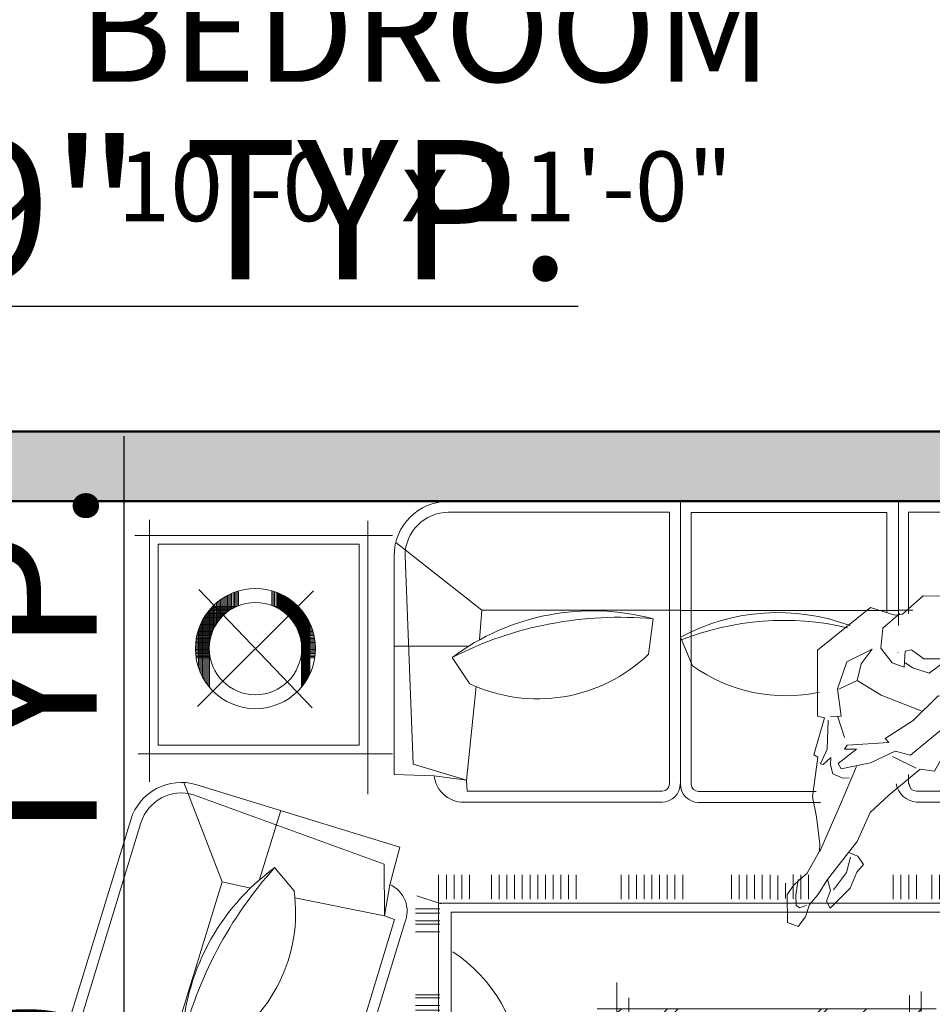
# Model space of a CAD drawing. Units: inches. Extents: x 375 to 1122, y 27 to 1069.
# Tile 75 of 155: x 509 to 588, y 792 to 877. Entities that reach past the tile are written whole.
import ezdxf

# ---------------------------------------------------------------- set-up
doc = ezdxf.new("R2010")
doc.units = ezdxf.units.IN
for name, color, linetype, lineweight in [('A-ANNO-DIMS', 2, 'Continuous', 18), ('A-AREA-IDEN', 7, 'Continuous', 18), ('A-WALL-PATT', 252, 'Continuous', 13), ('Furniture', 30, 'Continuous', 18), ('Walls', 250, 'Continuous', 50)]:
    doc.layers.add(name, color=color, linetype=linetype, lineweight=lineweight)
doc.styles.get("Standard").update_dxf_attribs({"font": 'arial.ttf'})
doc.dimstyles.new('ISO-25', dxfattribs={"dimtxt": 12, "dimasz": 2.5, "dimexe": 1.5, "dimexo": 1.5, "dimtad": 1, "dimdec": 1, "dimlunit": 3, "dimtxsty": 'Standard', "dimblk": 'ARCHTICK', "dimcen": 2.5, "dimadec": 0, "dimazin": 0, "dimtfac": 1, "dimtdec": 1, "dimtmove": 0, "dimatfit": 3, "dimfxl": 1.5, "dimfxlon": 1, "dimarcsym": 0})

# ---------------------------------------------------------------- blocks, each defined once
blk = doc.blocks.new('A$C4DC51D13')
for p, q in [((3265.3, 2996.2), (1188.4, 2996.2)), ((1895.2, 2134), (1895.2, 2996.2)), ((2559.6, 2996.2), (2559.6, 2617.8)), ((1188.4, 2962.7), (1862.1, 2962.7)), ((1862.1, 2134), (1862.1, 2962.7)), ((1928.3, 2961.6), (2524.2, 2961.6)), ((1928.3, 2134), (1928.3, 2961.6)), ((2524.2, 2961.6), (2524.2, 2658.6)), ((2590.4, 2962.7), (2590.4, 2654.5)), ((3265.3, 2962.7), (2590.4, 2962.7)), ((277.4, 2939.6), (277.4, 2141.8)), ((943, 2103.5), (943, 2936.7)), ((1018.2, 2892.3), (232.2, 2892.3)), ((3778.5, 2897), (3631.2, 2747.3)), ((4008.9, 2375.5), (3778.5, 2897)), ((4156.2, 2525.2), (3778.5, 2897)), ((304, 2865.7), (304, 2253.3)), ((916.4, 2865.7), (304, 2865.7)), ((916.4, 2253.3), (916.4, 2865.7)), ((1290.4, 2664.8), (1028, 2870.9)), ((3163.3, 2664.8), (3425.7, 2870.9)), ((1022.9, 2163.8), (1022.9, 2830.3)), ((1056, 2830.3), (1081, 2194.8)), ((3397.7, 2830.3), (3364.5, 2194.8)), ((3430.8, 2163.8), (3430.8, 2830.3)), ((4008.9, 2375.5), (3631.2, 2747.3)), ((423.7, 2370.8), (776.6, 2723.7)), ((427.4, 2727.4), (772.8, 2367.1)), ((502.2, 2648.3), (502.2, 2701.8)), ((506.4, 2652.2), (506.4, 2704.4)), ((510.6, 2655.8), (510.6, 2706.9)), ((514.9, 2659.2), (514.9, 2709.2)), ((519.1, 2662.3), (519.1, 2711.3)), ((523.3, 2665.1), (523.3, 2713.4)), ((527.5, 2667.8), (527.5, 2715.2)), ((531.8, 2670.2), (531.8, 2717)), ((536, 2672.5), (536, 2718.7)), ((540.2, 2674.6), (540.2, 2720.2)), ((544.4, 2676.5), (544.4, 2721.6)), ((548.7, 2678.2), (548.7, 2722.9)), ((650.1, 2678.8), (650.1, 2723.3)), ((654.3, 2677.1), (654.3, 2722)), ((658.6, 2675.2), (658.6, 2720.7)), ((662.8, 2673.2), (662.8, 2719.2)), ((667, 2671), (667, 2717.6)), ((668.5, 2670.2), (668.5, 2717)), ((671.2, 2668.6), (671.2, 2715.9)), ((672.7, 2667.8), (672.7, 2715.2)), ((675.5, 2666.1), (675.5, 2714)), ((676.9, 2665.1), (676.9, 2713.4)), ((679.7, 2663.3), (679.7, 2712)), ((681.1, 2662.3), (681.1, 2711.3)), ((683.9, 2660.3), (683.9, 2709.9)), ((685.4, 2659.2), (685.4, 2709.2)), ((688.1, 2657), (688.1, 2707.7)), ((689.6, 2655.8), (689.6, 2706.9)), ((692.4, 2653.5), (692.4, 2705.3)), ((693.8, 2652.2), (693.8, 2704.4)), ((696.6, 2649.6), (696.6, 2702.7)), ((698, 2648.3), (698, 2701.8)), ((700.8, 2645.5), (700.8, 2700)), ((465.8, 2671.5), (534.1, 2671.5)), ((468.4, 2596.6), (468.4, 2674.3)), ((469.8, 2675.7), (542.8, 2675.7)), ((472.6, 2606.7), (472.6, 2678.5)), ((476.8, 2615), (476.8, 2682.5)), ((481, 2622.2), (481, 2686.2)), ((485.3, 2628.5), (485.3, 2689.7)), ((489.5, 2634.2), (489.5, 2693)), ((493.7, 2639.3), (493.7, 2696.1)), ((497.9, 2644), (497.9, 2699.1)), ((657.4, 2675.7), (730.4, 2675.7)), ((734.5, 2671.5), (666.1, 2671.5)), ((666.1, 2671.5), (734.5, 2671.5)), ((702.3, 2644), (702.3, 2699.1)), ((705, 2641), (705, 2697.2)), ((706.5, 2639.3), (706.5, 2696.1)), ((709.3, 2636), (709.3, 2694.1)), ((710.7, 2634.2), (710.7, 2693)), ((713.5, 2630.5), (713.5, 2690.9)), ((714.9, 2628.5), (714.9, 2689.7)), ((717.7, 2624.4), (717.7, 2687.4)), ((719.2, 2622.2), (719.2, 2686.2)), ((722, 2617.6), (722, 2683.8)), ((723.4, 2615), (723.4, 2682.5)), ((726.2, 2609.7), (726.2, 2679.9)), ((727.6, 2606.7), (727.6, 2678.5)), ((730.4, 2600.3), (730.4, 2675.7)), ((731.9, 2596.6), (731.9, 2674.3)), ((734.6, 2588.4), (734.6, 2671.3)), ((3631.7, 2676.6), (3938.2, 2375)), ((443, 2453.4), (443, 2641.1)), ((443.5, 2641.9), (496, 2641.9)), ((446.1, 2646.1), (500, 2646.1)), ((447.2, 2446.7), (447.2, 2647.8)), ((448.9, 2650.4), (504.4, 2650.4)), ((451.5, 2440.6), (451.5, 2654)), ((451.9, 2654.6), (509.2, 2654.6)), ((455.1, 2658.8), (514.4, 2658.8)), ((455.7, 2434.9), (455.7, 2659.6)), ((458.4, 2663.1), (520.2, 2663.1)), ((459.9, 2558.8), (459.9, 2664.9)), ((462, 2667.3), (526.7, 2667.3)), ((464.1, 2583.3), (464.1, 2669.7)), ((489.5, 2667.3), (489.5, 2633.5)), ((738.2, 2667.3), (673.5, 2667.3)), ((673.5, 2667.3), (738.2, 2667.3)), ((741.8, 2663.1), (680, 2663.1)), ((680, 2663.1), (741.8, 2663.1)), ((745.2, 2658.8), (685.8, 2658.8)), ((685.8, 2658.8), (745.2, 2658.8)), ((748.3, 2654.6), (691, 2654.6)), ((691, 2654.6), (748.3, 2654.6)), ((751.3, 2650.4), (695.8, 2650.4)), ((695.8, 2650.4), (751.3, 2650.4)), ((754.1, 2646.1), (700.2, 2646.1)), ((700.2, 2646.1), (754.1, 2646.1)), ((756.7, 2641.9), (704.2, 2641.9)), ((704.2, 2641.9), (756.7, 2641.9)), ((736.1, 2583.3), (736.1, 2669.7)), ((738.9, 2570.4), (738.9, 2666.6)), ((740.3, 2558.8), (740.3, 2664.9)), ((743.1, 2433.1), (743.1, 2661.5)), ((744.5, 2434.9), (744.5, 2659.6)), ((747.3, 2438.6), (747.3, 2656)), ((748.8, 2440.6), (748.8, 2654)), ((751.5, 2444.5), (751.5, 2650)), ((753, 2446.7), (753, 2647.8)), ((755.8, 2451.1), (755.8, 2643.5)), ((757.2, 2453.4), (757.2, 2641.1)), ((1283.3, 2574.2), (1290.4, 2664.8)), ((1290.4, 2664.8), (1894.7, 2664.8)), ((1895.2, 2663.7), (2557.3, 2663.7)), ((2603.6, 2664.8), (2559, 2664.8)), ((3163.3, 2664.8), (2764.7, 2664.8)), ((3170.4, 2574.2), (3163.3, 2664.8)), ((429.1, 2612.3), (475.4, 2612.3)), ((430.3, 2479), (430.3, 2615.5)), ((430.7, 2616.6), (477.7, 2616.6)), ((432.5, 2620.8), (480.2, 2620.8)), ((434.5, 2469.3), (434.5, 2625.2)), ((434.5, 2625), (482.9, 2625)), ((436.5, 2629.2), (485.8, 2629.2)), ((438.7, 2633.5), (488.9, 2633.5)), ((438.8, 2460.9), (438.8, 2633.6)), ((441, 2637.7), (492.3, 2637.7)), ((759.2, 2637.7), (707.9, 2637.7)), ((707.9, 2637.7), (759.2, 2637.7)), ((761.5, 2633.5), (711.3, 2633.5)), ((711.3, 2633.5), (761.5, 2633.5)), ((763.7, 2629.2), (714.4, 2629.2)), ((714.4, 2629.2), (763.7, 2629.2)), ((765.8, 2625), (717.3, 2625)), ((767.7, 2620.8), (720, 2620.8)), ((769.5, 2616.6), (722.5, 2616.6)), ((771.1, 2612.3), (724.8, 2612.3)), ((760, 2458.3), (760, 2636.3)), ((761.4, 2460.9), (761.4, 2633.6)), ((764.2, 2466.3), (764.2, 2628.2)), ((765.7, 2469.3), (765.7, 2625.2)), ((1798, 2530.2), (1812.1, 2637.9)), ((420.6, 2582.7), (464, 2582.7)), ((421.5, 2587), (465.2, 2587)), ((422.5, 2591.2), (466.5, 2591.2)), ((423.6, 2595.4), (467.9, 2595.4)), ((424.8, 2599.7), (469.6, 2599.7)), ((426.1, 2603.9), (471.3, 2603.9)), ((426.1, 2490.7), (426.1, 2603.9)), ((427.5, 2608.1), (473.3, 2608.1)), ((772.7, 2608.1), (726.9, 2608.1)), ((774.1, 2603.9), (728.9, 2603.9)), ((775.4, 2599.7), (730.7, 2599.7)), ((776.6, 2595.4), (732.3, 2595.4)), ((777.7, 2591.2), (733.7, 2591.2)), ((778.7, 2587), (735.1, 2587)), ((779.6, 2582.7), (736.2, 2582.7)), ((1895.5, 2582.2), (1932.3, 2494.6)), ((417.2, 2553.2), (459.6, 2553.2)), ((417.4, 2557.4), (459.8, 2557.4)), ((417.7, 2561.6), (460.2, 2561.6)), ((418.1, 2565.8), (460.7, 2565.8)), ((418.5, 2570.1), (461.3, 2570.1)), ((419.1, 2574.3), (462.1, 2574.3)), ((419.8, 2578.5), (462.9, 2578.5)), ((780.4, 2578.5), (737.3, 2578.5)), ((781.1, 2574.3), (738.2, 2574.3)), ((781.7, 2570.1), (738.9, 2570.1)), ((782.2, 2565.8), (739.6, 2565.8)), ((782.5, 2561.6), (740.1, 2561.6)), ((782.8, 2557.4), (740.4, 2557.4)), ((783, 2553.2), (740.7, 2553.2)), ((1022.9, 2554.4), (1249.6, 2554.4)), ((3430.8, 2554.4), (3204.1, 2554.4)), ((417.1, 2548.9), (459.4, 2548.9)), ((417.1, 2544.7), (459.5, 2544.7)), ((417.2, 2540.5), (459.6, 2540.5)), ((417.5, 2536.3), (459.9, 2536.3)), ((417.8, 2532), (460.3, 2532)), ((418.2, 2527.8), (460.8, 2527.8)), ((418.7, 2523.6), (461.4, 2523.6)), ((459.9, 2429.7), (459.9, 2535.7)), ((781.6, 2523.6), (738.8, 2523.6)), ((782.1, 2527.8), (739.4, 2527.8)), ((782.5, 2532), (740, 2532)), ((740.3, 2429.7), (740.3, 2535.7)), ((782.8, 2536.3), (740.4, 2536.3)), ((783, 2540.5), (740.6, 2540.5)), ((783.1, 2548.9), (740.8, 2548.9)), ((783.1, 2544.7), (740.8, 2544.7)), ((1200, 2520.5), (1251.9, 2440.8)), ((2559, 2535.8), (2557.3, 2535.8)), ((3253.7, 2520.5), (3201.8, 2440.8)), ((4008.9, 2375.5), (4156.2, 2525.2)), ((419.3, 2519.4), (462.2, 2519.4)), ((781, 2519.4), (738, 2519.4)), ((1243.2, 2146.7), (1272.2, 2431.8)), ((3210.5, 2146.7), (3181.5, 2431.8)), ((304, 2253.3), (916.4, 2253.3)), ((242.9, 2226.7), (1018.2, 2226.7)), ((1081, 2194.8), (1243.2, 2146.7)), ((3364.5, 2194.8), (3210.5, 2146.7)), ((1145.1, 2159.3), (1022.9, 2163.8)), ((2590.4, 2164.3), (2590.4, 2134)), ((3308.6, 2159.3), (3430.8, 2163.8)), ((498.8, 1837.1), (382.1, 2139.5)), ((1040.3, 1942.9), (421.2, 2132.6)), ((1145.1, 2159.3), (1243.2, 2146.7)), ((1244.8, 2113), (1243.2, 2146.7)), ((3208.9, 2113), (3210.5, 2146.7)), ((3308.6, 2159.3), (3210.5, 2146.7)), ((411.8, 2101.9), (992.6, 1890.2)), ((1839.5, 2113), (1244.8, 2113)), ((2308.5, 2111.9), (1950.4, 2111.9)), ((2614.2, 2113), (3208.9, 2113)), ((1839.5, 2079.9), (1244.8, 2079.9)), ((2322.1, 2078.8), (1950.4, 2078.8)), ((2614.2, 2079.9), (3208.9, 2079.9)), ((677.4, 2054.1), (612.9, 1843.6)), ((220.3, 2026), (19.3, 1370.1)), ((251.1, 2016.6), (37.1, 1314.7)), ((1009.7, 1828.1), (1040.3, 1942.9)), ((992.6, 1890.2), (993.4, 1733.4)), ((658.5, 1880), (717.8, 1809.1)), ((498.8, 1837.1), (341.4, 1323.6)), ((584.9, 1817.9), (498.8, 1837.1)), ((1158.3, 1784.3), (1158.3, 1858.2)), ((1181.8, 1784.3), (1181.8, 1858.2)), ((1205.3, 1784.3), (1205.3, 1858.2)), ((1228.8, 1784.3), (1228.8, 1858.2)), ((1252.2, 1784.3), (1252.2, 1858.2)), ((1319.4, 1784.3), (1319.4, 1858.2)), ((1342.9, 1784.3), (1342.9, 1858.2)), ((1366.3, 1784.3), (1366.3, 1858.2)), ((1389.8, 1784.3), (1389.8, 1858.2)), ((1413.3, 1784.3), (1413.3, 1858.2)), ((1436.8, 1784.3), (1436.8, 1858.2)), ((1460.2, 1784.3), (1460.2, 1858.2)), ((1483.7, 1784.3), (1483.7, 1858.2)), ((1507.2, 1784.3), (1507.2, 1858.2)), ((1530.7, 1784.3), (1530.7, 1858.2)), ((1554.1, 1784.3), (1554.1, 1858.2)), ((1577.6, 1784.3), (1577.6, 1858.2)), ((1714.2, 1784.3), (1714.2, 1858.2)), ((1737.6, 1784.3), (1737.6, 1858.2)), ((1761.1, 1784.3), (1761.1, 1858.2)), ((1784.6, 1784.3), (1784.6, 1858.2)), ((1808.1, 1784.3), (1808.1, 1858.2)), ((1831.5, 1784.3), (1831.5, 1858.2)), ((1855, 1784.3), (1855, 1858.2)), ((1878.5, 1784.3), (1878.5, 1858.2)), ((1902, 1784.3), (1902, 1858.2)), ((2050.7, 1784.3), (2050.7, 1858.2)), ((2074.2, 1784.3), (2074.2, 1858.2)), ((2097.7, 1784.3), (2097.7, 1858.2)), ((2121.1, 1784.3), (2121.1, 1858.2)), ((2144.6, 1784.3), (2144.6, 1858.2)), ((2168.1, 1784.3), (2168.1, 1858.2)), ((2191.6, 1782.4), (2191.6, 1856.3)), ((2215, 1785.7), (2215, 1832.3)), ((2238.5, 1785.1), (2238.5, 1859)), ((2262, 1784.3), (2262, 1858.2)), ((2285.4, 1784.3), (2285.4, 1858.2)), ((2543.7, 1784.3), (2543.7, 1858.2)), ((2567.1, 1784.3), (2567.1, 1858.2)), ((2590.6, 1784.3), (2590.6, 1858.2)), ((2614.1, 1784.3), (2614.1, 1858.2)), ((2661, 1784.3), (2661, 1858.2)), ((2684.5, 1784.3), (2684.5, 1858.2)), ((2708, 1772.3), (2708, 1858.2)), ((2731.5, 1784.3), (2731.5, 1858.2)), ((2754.9, 1784.3), (2754.9, 1858.2)), ((2778.4, 1784.3), (2778.4, 1858.2)), ((2801.9, 1784.3), (2801.9, 1858.2)), ((2825.4, 1784.3), (2825.4, 1858.2)), ((2848.8, 1784.3), (2848.8, 1858.2)), ((2872.3, 1784.3), (2872.3, 1858.2)), ((2895.8, 1784.3), (2895.8, 1858.2)), ((2919.3, 1784.3), (2919.3, 1858.2)), ((2942.7, 1784.3), (2942.7, 1858.2)), ((2966.2, 1744.8), (2966.2, 1858.2)), ((2989.7, 1784.3), (2989.7, 1858.2)), ((3013.2, 1772.3), (3013.2, 1858.2)), ((3036.6, 1784.3), (3036.6, 1858.2)), ((3060.1, 1784.3), (3060.1, 1858.2)), ((3083.6, 1784.3), (3083.6, 1858.2)), ((1009.7, 1828.1), (993.4, 1733.4)), ((1158.3, 1821.3), (1158.5, 487.7)), ((993.4, 1733.4), (720.4, 1787.6)), ((1166.1, 1769.7), (1091.8, 1794.5)), ((3248.4, 1772.3), (1158.5, 1772.3)), ((3248.4, 487.7), (3248.4, 1772.3)), ((1162.1, 1754.9), (1088.2, 1754.9)), ((1162.1, 1741.1), (1088.2, 1741.1)), ((1196, 511), (1196, 1744.8)), ((1196, 1744.8), (3215.6, 1744.8)), ((3215.6, 511), (3215.6, 1744.8)), ((3248.8, 1760.8), (3322.7, 1760.8)), ((3600.6, 1621.7), (3605.1, 1743.8)), ((3605.1, 1743.8), (4271.6, 1743.8)), ((3995.7, 1743.8), (3995.7, 1517.1)), ((1024.2, 1722.3), (842.3, 1125.2)), ((873.1, 1115.8), (1055, 1712.9)), ((1024.2, 1722.3), (993.4, 1733.4)), ((1162.1, 1717.6), (1088.2, 1717.6)), ((3248.8, 1737.3), (3322.7, 1737.3)), ((3248.8, 1713.8), (3322.7, 1713.8)), ((4271.6, 1710.7), (3636.1, 1685.8)), ((4106.1, 1476.4), (4312.2, 1738.8)), ((1162.1, 1708), (1088.2, 1708)), ((1162.1, 1684.5), (1088.2, 1684.5)), ((3248.8, 1690.4), (3322.7, 1690.4)), ((3636.1, 1685.8), (3588, 1523.6)), ((3248.8, 1666.9), (3322.7, 1666.9)), ((3248.8, 1643.4), (3322.7, 1643.4)), ((3248.8, 1619.9), (3322.7, 1619.9)), ((3600.6, 1621.7), (3588, 1523.6)), ((4404, 1578.3), (4404, 904.6)), ((4437.5, 165.9), (4437.5, 1578.3)), ((1701.7, 1530), (1701.7, 911.2)), ((2629.1, 907.9), (2629.1, 1503.1)), ((3248.8, 1513.8), (3322.7, 1513.8)), ((3248.8, 1513.3), (3322.7, 1513.3)), ((3521.2, 1130.7), (3521.2, 1521.9)), ((3554.3, 1131.4), (3554.3, 1521.9)), ((3588, 1523.6), (3873.1, 1494.5)), ((1162.1, 1492.9), (1088.2, 1492.9)), ((1162.1, 1483.3), (1088.2, 1483.3)), ((1737.7, 1483.1), (1737.7, 911.2)), ((2593.1, 907.9), (2593.1, 1490.3)), ((3248.8, 1490.4), (3322.7, 1490.4)), ((3248.8, 1489.9), (3322.7, 1489.9)), ((4015.5, 1483.4), (4106.1, 1476.4)), ((4106.1, 1476.4), (4106.1, 872.1)), ((1162.1, 1459.8), (1088.2, 1459.8)), ((1162.1, 1446), (1088.2, 1446)), ((2674.6, 1449.9), (1641, 1449.9)), ((1888.1, 1449.9), (1701.7, 1263.5)), ((1856.2, 1449.9), (1701.7, 1295.4)), ((1715.1, 1449.9), (1701.7, 1436.5)), ((2343.3, 1449.9), (1855.3, 961.9)), ((2629.1, 1449), (2142, 961.9)), ((2325.1, 1449.9), (2154.2, 1279.1)), ((2461.6, 1449.9), (2177, 1165.3)), ((3248.8, 1466.9), (3322.7, 1466.9)), ((3248.8, 1443.4), (3322.7, 1443.4)), ((1162.1, 1412.8), (1088.2, 1412.8)), ((2674.6, 1413.9), (1641, 1413.9)), ((3248.8, 1419.9), (3322.7, 1419.9)), ((1162.1, 1399), (1088.2, 1399)), ((3250, 1407.8), (3519, 1407.8)), ((6.3, 1324.2), (19.3, 1370.2)), ((1162.1, 1375.5), (1088.2, 1375.5)), ((1162.1, 1352.1), (1088.2, 1352.1)), ((3248.8, 1359), (3322.7, 1359)), ((342.8, 1324.6), (76.7, 1139.6)), ((843, 1127.6), (342.8, 1324.6)), ((479.3, 1327.3), (375.2, 1344.9)), ((1162.1, 1342.9), (1088.2, 1342.9)), ((1162.1, 1342.4), (1088.2, 1342.4)), ((3248.8, 990.8), (3248.4, 1328.4)), ((1162.1, 1319.4), (1088.2, 1319.4)), ((1162.1, 1318.9), (1088.2, 1318.9)), ((1162.1, 1296), (1088.2, 1296)), ((1162.1, 1295.5), (1088.2, 1295.5)), ((3248.8, 1312.1), (3322.7, 1312.1)), ((3248.8, 1302.3), (3322.7, 1302.3)), ((3250, 1317.8), (3519, 1317.8)), ((369.2, 1044.8), (442.9, 1285.2)), ((1196, 1272.5), (1088.2, 1272.5)), ((1162.1, 1272), (1088.2, 1272)), ((2629.1, 1280.5), (2310.5, 961.9)), ((1162.1, 1249), (1088.2, 1249)), ((1162.1, 1248.5), (1088.2, 1248.5)), ((3248.8, 1249), (3322.7, 1249)), ((3248.8, 1248.5), (3322.7, 1248.5)), ((3248.8, 1239.3), (3322.7, 1239.3)), ((3248.8, 1238.8), (3322.7, 1238.8)), ((1162.1, 1225.5), (1088.2, 1225.5)), ((1162.1, 1202.1), (1088.2, 1202.1)), ((3248.8, 1225.5), (3322.7, 1225.5)), ((3248.8, 1202.1), (3322.7, 1202.1)), ((1196, 1178.6), (1088.2, 1178.6)), ((3248.8, 1178.6), (3322.7, 1178.6)), ((122.4, 1154.1), (719.7, 996.3)), ((1162.1, 1155.1), (1088.2, 1155.1)), ((1728.6, 1158.4), (1701.7, 1131.5)), ((3248.8, 1155.1), (3322.7, 1155.1)), ((732, 933.5), (112.9, 1123.3)), ((719.7, 996.3), (810.6, 1133.2)), ((771, 1045.7), (810.6, 1133.2)), ((842.3, 1125.2), (810.6, 1133.2)), ((1162.1, 1131.6), (1088.2, 1131.6)), ((3248.8, 1131.6), (3322.7, 1131.6)), ((1162.1, 1108.2), (1088.2, 1108.2)), ((1162.1, 1084.7), (1088.2, 1084.7)), ((3248.8, 1108.2), (3322.7, 1108.2)), ((1196, 1061.2), (1088.2, 1061.2)), ((1926.6, 1051.5), (1837.1, 961.9)), ((771, 1045.7), (732, 933.5)), ((1162.1, 1037.7), (1088.2, 1037.7)), ((1162.1, 1014.3), (1088.2, 1014.3)), ((1648.3, 1019.6), (2616.7, 1019.6)), ((2006.3, 994.6), (1973.6, 961.9)), ((2629.1, 1012), (2579, 961.9)), ((3248.8, 1014.3), (3322.7, 1014.3)), ((3248.8, 990.8), (3322.7, 990.8)), ((1196, 967.3), (1088.2, 967.3)), ((1648.3, 961.9), (2681.9, 961.9)), ((2459.2, 974.1), (2447, 961.9)), ((3248.8, 967.3), (3322.7, 967.3)), ((1162.1, 943.8), (1088.2, 943.8)), ((3248.8, 943.8), (3322.7, 943.8)), ((1162.1, 920.4), (1088.2, 920.4)), ((3248.8, 920.4), (3322.7, 920.4)), ((4097.4, 904.6), (4404, 904.6)), ((4106.1, 871.5), (4437.5, 871.5)), ((1196, 860.5), (1088.2, 860.5)), ((4404, 840.7), (4110.5, 840.7)), ((4404, 165.9), (4404, 840.7)), ((1162.1, 837), (1088.2, 837)), ((1162.1, 813.5), (1088.2, 813.5)), ((3521.2, 816.9), (3521.2, 222.3)), ((3554.3, 816.9), (3554.3, 222.3)), ((1162.1, 790), (1031.8, 790)), ((1196, 766.6), (1088.2, 766.6)), ((1162.1, 743.1), (1088.2, 743.1)), ((1162.1, 719.6), (1088.2, 719.6)), ((4106.1, 267.8), (4106.1, 666.5)), ((1162.1, 627.8), (1088.2, 627.8)), ((1162.1, 604.4), (1088.2, 604.4)), ((3248.8, 627.8), (3322.7, 627.8)), ((3248.8, 604.4), (3322.7, 604.4)), ((1162.1, 580.9), (1034.2, 580.9)), ((3248.8, 580.9), (3322.7, 580.9)), ((1162.1, 557.4), (1088.2, 557.4)), ((3248.8, 557.4), (3322.7, 557.4)), ((1162.1, 533.9), (1088.2, 533.9)), ((1162.1, 510.5), (1088.2, 510.5)), ((3215.6, 511), (1196, 511)), ((1334.6, 511), (1334.6, 402.4)), ((1381.6, 511), (1381.6, 402.4)), ((2059.5, 511), (2059.5, 402.4)), ((2106.4, 511), (2106.4, 402.4)), ((2669.8, 511), (2669.8, 402.4)), ((3248.8, 533.9), (3322.7, 533.9)), ((3248.8, 510.5), (3322.7, 510.5)), ((1162, 495.1), (1116.6, 429)), ((1158.5, 487.7), (3248.4, 487.7)), ((1311.1, 487.7), (1311.1, 402.4)), ((1428.5, 487.7), (1428.5, 402.4)), ((1498.9, 487.7), (1498.9, 402.4)), ((1522.4, 487.7), (1522.4, 402.4)), ((1663.3, 487.7), (1663.3, 402.4)), ((1757.8, 487.7), (1757.8, 402.4)), ((1781.3, 487.7), (1781.3, 402.4)), ((1922.1, 487.7), (1922.1, 402.4)), ((2036, 487.7), (2036, 402.4)), ((2153.4, 487.7), (2153.4, 402.4)), ((2223.8, 487.7), (2223.8, 402.4)), ((2247.2, 487.7), (2247.2, 402.4)), ((2388.1, 487.7), (2388.1, 402.4)), ((2482, 487.7), (2482, 402.4)), ((2505.5, 487.7), (2505.5, 402.4)), ((2740.2, 487.7), (2740.2, 402.4)), ((2784.9, 487.7), (2784.9, 402.4)), ((2904.5, 487.7), (2904.5, 402.4)), ((3021.9, 487.7), (3021.9, 402.4)), ((3092.7, 484.5), (3092.7, 410.6)), ((3116.2, 484.5), (3116.2, 410.6)), ((3244.9, 495.1), (3290.3, 429)), ((1167.1, 476.3), (1167.1, 402.4)), ((1190.6, 476.3), (1190.6, 402.4)), ((1214, 476.3), (1214, 402.4)), ((1237.5, 476.3), (1237.5, 402.4)), ((1358.1, 476.3), (1358.1, 402.4)), ((1405, 476.3), (1405, 402.4)), ((1452, 476.3), (1452, 402.4)), ((1475.5, 476.3), (1475.5, 402.4)), ((1545.9, 476.3), (1545.9, 402.4)), ((1569.4, 476.3), (1569.4, 402.4)), ((1592.8, 476.3), (1592.8, 402.4)), ((1616.3, 476.3), (1616.3, 402.4)), ((1639.8, 476.3), (1639.8, 402.4)), ((1804.8, 476.3), (1804.8, 402.4)), ((1828.2, 476.3), (1828.2, 402.4)), ((1851.7, 476.3), (1851.7, 402.4)), ((1875.2, 476.3), (1875.2, 402.4)), ((1898.7, 476.3), (1898.7, 402.4)), ((2082.9, 476.3), (2082.9, 402.4)), ((2129.9, 476.3), (2129.9, 402.4)), ((2176.8, 476.3), (2176.8, 402.4)), ((2200.3, 476.3), (2200.3, 402.4)), ((2270.7, 476.3), (2270.7, 402.4)), ((2294.2, 476.3), (2294.2, 402.4)), ((2317.7, 476.3), (2317.7, 402.4)), ((2341.1, 476.3), (2341.1, 402.4)), ((2364.6, 476.3), (2364.6, 402.4)), ((2411.6, 476.3), (2411.6, 402.4)), ((2435, 476.3), (2435, 402.4)), ((2458.5, 476.3), (2458.5, 402.4)), ((2528.9, 476.3), (2528.9, 402.4)), ((2552.4, 476.3), (2552.4, 402.4)), ((2575.9, 476.3), (2575.9, 402.4)), ((2599.4, 476.3), (2599.4, 402.4)), ((2622.8, 476.3), (2622.8, 402.4)), ((2646.3, 476.3), (2646.3, 402.4)), ((2693.3, 476.3), (2693.3, 402.4)), ((2716.7, 476.3), (2716.7, 402.4)), ((2738, 476.3), (2738, 402.4)), ((2761.5, 476.3), (2761.5, 402.4)), ((2763.7, 476.3), (2763.7, 402.4)), ((2787.2, 476.3), (2787.2, 402.4)), ((2808.4, 476.3), (2808.4, 402.4)), ((2810.6, 476.3), (2810.6, 402.4)), ((2831.9, 476.3), (2831.9, 402.4)), ((2834.1, 476.3), (2834.1, 402.4)), ((2855.4, 476.3), (2855.4, 402.4)), ((2857.6, 476.3), (2857.6, 402.4)), ((2878.8, 476.3), (2878.8, 402.4)), ((2881.1, 476.3), (2881.1, 402.4)), ((2902.3, 476.3), (2902.3, 402.4)), ((2925.8, 476.3), (2925.8, 402.4)), ((2928, 476.3), (2928, 402.4)), ((2949.3, 476.3), (2949.3, 402.4)), ((2951.5, 476.3), (2951.5, 402.4)), ((2972.7, 476.3), (2972.7, 402.4)), ((2975, 476.3), (2975, 402.4)), ((2996.2, 476.3), (2996.2, 402.4)), ((2998.4, 476.3), (2998.4, 402.4)), ((3019.7, 476.3), (3019.7, 402.4)), ((3043.2, 476.3), (3043.2, 402.4)), ((3045.4, 476.3), (3045.4, 402.4)), ((3066.6, 476.3), (3066.6, 402.4)), ((3068.9, 476.3), (3068.9, 402.4)), ((3092.3, 476.3), (3092.3, 402.4)), ((3115.8, 476.3), (3115.8, 402.4)), ((3202.2, 476.3), (3202.2, 402.4)), ((3225.7, 476.3), (3225.7, 402.4)), ((3249.2, 476.3), (3249.2, 402.4)), ((3588, 220.6), (3873.1, 249.7)), ((4015.5, 260.8), (4106.1, 267.8)), ((4106.1, 267.8), (4312.2, 5.4)), ((3636.1, 66.6), (3588, 220.6)), ((3961.8, 177.4), (3882.1, 229.3)), ((3995.7, 0.4), (3995.7, 227)), ((3600.6, 122.5), (3605.1, 0.4)), ((4271.6, 33.5), (3636.1, 66.6)), ((3605.1, 0.4), (4271.6, 0.4))]:
    blk.add_line(p, q)
at = {"linetype": 'ByBlock'}
for points in [[(2342.9, 1843.9), (2352.5, 1810.4), (2340.1, 1777.7), (2351.8, 1757), (2412.3, 1818), (2433.1, 1866.4), (2453.1, 1889.5), (2436, 1914.7), (2407.6, 1926.2), (2433.7, 1959.9), (2473.1, 2048.3), (2530.6, 2101.1), (2625.9, 2180.3), (2669, 2174.2), (2748.1, 2315.4), (2745.8, 2342.6), (2801.2, 2404.9), (2823.9, 2479.6), (2818.4, 2529.9), (2775.1, 2571.7), (2782.4, 2583.3), (2765.2, 2658.8), (2714.5, 2706.9), (2634.6, 2708.6), (2571.9, 2652.6), (2548.8, 2649.4), (2474, 2672.1), (2312.9, 2542.1), (2312.9, 2341.6), (2333.9, 2336.4), (2302, 2223.9), (2313.6, 2216.6), (2297.4, 2095.7), (2309.3, 2034.9), (2320.2, 1952), (2319.3, 1929.9), (2280.8, 1863.6), (2257.7, 1842.4), (2239.2, 1825.7), (2220.1, 1798.2), (2221.6, 1713.1), (2254.3, 1700.7), (2275.9, 1729.8), (2288.6, 1768), (2313.7, 1797.6)], [(3285.2, 1088.3), (3251.7, 1078.6), (3219, 1091.1), (3198.3, 1079.4), (3259.3, 1018.8), (3307.7, 998), (3330.8, 978), (3356, 995.1), (3367.5, 1023.6), (3401.2, 997.5), (3489.6, 958), (3542.4, 900.5), (3621.6, 805.3), (3615.5, 762.2), (3756.7, 683), (3783.9, 685.3), (3846.2, 629.9), (3920.9, 607.2), (3971.2, 612.7), (4013, 656), (4024.6, 648.7), (4100.1, 665.9), (4148.2, 716.6), (4149.9, 796.5), (4093.9, 859.3), (4090.7, 882.4), (4113.4, 957.1), (3983.4, 1118.2), (3782.9, 1118.2), (3777.7, 1097.2), (3665.2, 1129.2), (3657.9, 1117.6), (3537, 1133.7), (3476.2, 1121.9), (3393.3, 1110.9), (3371.2, 1111.9), (3304.9, 1150.4), (3283.7, 1173.4), (3267, 1191.9), (3239.5, 1211), (3154.4, 1209.5), (3142, 1176.8), (3171.1, 1155.3), (3209.3, 1142.5), (3238.9, 1117.5)]]:
    blk.add_lwpolyline(points, close=True, dxfattribs=at)
for points in [[(2563.4, 2654.7), (2512.2, 2609.3), (2506.2, 2548.3), (2540.1, 2504.4), (2576.9, 2490.9), (2579.8, 2539.3), (2598.7, 2543.6), (2636.7, 2516.4), (2690.3, 2516.7), (2731.2, 2520.1), (2758.5, 2540.1), (2773, 2563.3)], [(2629.1, 2357.8), (2507, 2405.5), (2433.2, 2450.3), (2445.5, 2500.8), (2478.9, 2546.1), (2402.4, 2506.9), (2373.4, 2424.8), (2384.4, 2341.9), (2352.8, 2340.7)], [(2712.3, 2515.8), (2652.7, 2472.4), (2603.2, 2489), (2580, 2503.6)], [(2738, 2438.2), (2699.2, 2425.4), (2742.4, 2401.4), (2680.4, 2403.2), (2604.1, 2328.3), (2519.2, 2273.3), (2529.8, 2261.8), (2402.7, 2252.7), (2395.4, 2241.1), (2431.1, 2241.3), (2375.7, 2196.9), (2385.2, 2181.2), (2474.4, 2199.5), (2549.9, 2234.6), (2596.2, 2223.2), (2730.1, 2333.1)], [(2433.2, 2450.3), (2377.6, 2423.8)], [(2409.5, 2153), (2387.5, 2153.9), (2359, 2165.4), (2352.6, 2193.7), (2353.5, 2215.7), (2330.5, 2194.6), (2322.1, 2196.7), (2341.8, 2240.9), (2345.5, 2329.1)], [(2374.9, 2339.8), (2395.2, 2276.9)], [(2613.2, 2183.4), (2541.6, 2218.8)], [(2431.4, 2187.8), (2379.5, 2066.7), (2320.2, 1929.7)], [(2407.6, 1926.2), (2342.9, 1843.9)], [(2412.9, 1911.5), (2401.6, 1865.2), (2361.9, 1812.5)], [(2279.2, 1765.9), (2259.2, 1757.4), (2247.6, 1764.7), (2246.4, 1796.2), (2253.5, 1843.5)], [(3207.2, 1152), (3198.7, 1171.9), (3206, 1183.5), (3237.5, 1184.7), (3284.8, 1177.6)], [(3629.1, 999.7), (3508, 1051.6), (3371, 1110.9)], [(3367.5, 1023.6), (3285.2, 1088.3)], [(3594.3, 1021.6), (3595.2, 1043.7), (3606.7, 1072.1), (3635, 1078.6), (3657, 1077.6), (3635.9, 1100.6), (3638, 1109.1), (3682.2, 1089.3), (3770.4, 1085.6)], [(3352.8, 1018.2), (3306.5, 1029.5), (3253.8, 1069.2)], [(3879.5, 693.2), (3866.7, 732), (3842.7, 688.8), (3844.5, 750.8), (3769.6, 827.1), (3714.6, 911.9), (3703.1, 901.3), (3694, 1028.4), (3682.4, 1035.7), (3682.6, 1000), (3638.2, 1055.5), (3622.5, 1045.9), (3640.8, 956.7), (3675.9, 881.2), (3664.5, 834.9), (3774.4, 701)], [(3781.1, 1056.2), (3718.2, 1035.9)], [(3799.1, 802), (3846.8, 924.2), (3891.6, 998), (3942.1, 985.6), (3987.4, 952.2), (3948.2, 1028.7), (3866.1, 1057.7), (3783.2, 1046.8), (3782, 1078.3)], [(3891.6, 998), (3865.1, 1053.5)], [(4096, 867.7), (4050.6, 918.9), (3989.6, 924.9), (3945.7, 891.1), (3932.2, 854.2), (3980.6, 851.3), (3984.9, 832.4), (3957.7, 794.4), (3958, 740.9), (3961.4, 699.9), (3981.4, 672.7), (4004.6, 658.1)], [(3624.7, 817.9), (3660.1, 889.6)], [(3957.1, 718.8), (3913.7, 778.5), (3930.3, 827.9), (3944.9, 851.1)]]:
    blk.add_lwpolyline(points, dxfattribs=at)
for centre, radius in [((600.1, 2547.3), 183), ((600.1, 2547.3), 140.7), ((1803.2, 1372.6), 25.7), ((2527.6, 1372.6), 25.7), ((1803.2, 1039.3), 25.7), ((2527.6, 1039.3), 25.7), ((2817.9, 923.4), 31.7), ((2095.7, 858), 41)]:
    blk.add_circle(centre, radius)
for centre, radius, start, end in [((1188.4, 2830.3), 165.9, 90, 180), ((3265.3, 2830.3), 165.9, 0, 90), ((1188.4, 2830.3), 132.4, 90, 180), ((3265.3, 2830.3), 132.4, 0, 90), ((3666.8, 2712.2), 50, 135.4503, 225.4503), ((1626.8, 1949.8), 712.7, 74.928, 126.7929), ((1707.9, 1527), 1115.8, 84.6406, 117.0804), ((2192.2, 2032.6), 624.6, 69.4145, 118.3621), ((2633.9, 373.6), 2292.5, 91.8726, 91.9144), ((2832.8, 1963.1), 698.5, 52.9389, 95.0789), ((2210.2, 1780.8), 852.5, 76.866, 111.6839), ((2713.3, 1357.7), 1282.3, 65.0725, 87.2152), ((1459.9, 2882.7), 488.4, 244.7866, 313.8058), ((2216, 2892.1), 488.4, 234.4888, 282.1285), ((2993.8, 2882.7), 488.4, 248.2152, 295.2134), ((3973.2, 2410.6), 50, 225.4503, 315.4503), ((374.1, 1978.9), 160.8, 72.9571, 162.9571), ((1234.5, 2169.3), 90, 186.4251, 276.5821), ((1839.5, 2135.1), 22.1, 270, 0), ((1839.5, 2135.1), 55.2, 270, 0), ((1950.4, 2134), 55.2, 180, 270), ((1950.4, 2134), 22.1, 180, 270), ((2619.6, 2148.3), 68.5, 191.0595, 265.4426), ((2614.2, 2135.1), 22.1, 180, 270), ((3219.2, 2169.3), 90, 263.4179, 353.5749), ((374.1, 1978.9), 128.6, 72.9571, 162.9571), ((1584.7, 1047), 1245.7, 138.0296, 166.1636), ((1067.1, 1321), 692.3, 126.1642, 178.0291), ((248.2, 1741.7), 474.4, 299.1514, 8.1705), ((974.8, 1747.9), 87.4, 336.375, 66.532), ((4271.6, 1578.3), 165.9, 0, 90), ((4271.6, 1578.3), 132.4, 0, 90), ((944.2, 1233.8), 467.1, 309.4804, 56.621), ((3610.6, 1532.2), 90, 96.4251, 186.5821), ((3383, 1136.2), 721.4, 348.1046, 36.6442), ((2968.3, 1058.8), 1115.8, 356.7543, 27.0804), ((4324, 1306.8), 488.4, 154.7866, 202.7137), ((160.1, 1277), 160.8, 162.9571, 252.9571), ((160.1, 1277), 128.6, 162.9571, 252.9571), ((2517.5, 1143.6), 586.7, 287.3395, 13.1463), ((787.1, 1131.7), 87.4, 259.3822, 349.5393), ((2356.9, 1798.1), 1287.8, 212.1153, 261.9323), ((-29968.2, -49615.7), 59944, 56.743614, 57.623407), ((3404.4, 598.4), 698.5, 322.9389, 5.0789), ((2799, 717.9), 1282.3, 335.0725, 357.2152), ((4324, 437.4), 488.4, 158.2152, 205.2134), ((2591.9, -2109.1), 2694.5, 80.9842, 100.0261), ((3610.6, 212), 90, 173.4179, 263.5749), ((4271.6, 165.9), 132.4, 270, 0), ((4271.6, 165.9), 165.9, 270, 0)]:
    blk.add_arc(centre, radius, start, end)
blk = doc.blocks.new('_ArchTick')
at = {"color": 0, "linetype": 'ByBlock', "const_width": 0.15}
blk.add_lwpolyline([(-0.5, -0.5), (0.5, 0.5)], dxfattribs=at)
blk = doc.blocks.new('*D48')
at = {"layer": 'A-ANNO-DIMS', "color": 0, "lineweight": -2, "transparency": 16777216}
for p, q in [((471.507, 853.828), (471.507, 850.828)), ((480.507, 853.828), (480.507, 850.828)), ((471.507, 852.328), (480.507, 852.328)), ((480.507, 852.328), (557.403, 852.328))]:
    blk.add_line(p, q, dxfattribs=at)
at = {"layer": 'Defpoints', "color": 0, "transparency": 16777216}
for p in [(471.507, 859.528), (480.507, 859.528), (480.507, 852.328)]:
    blk.add_point(p, dxfattribs=at)
at = {"layer": 'A-ANNO-DIMS', "color": 0, "lineweight": -2, "transparency": 16777216, "xscale": 2.5, "yscale": 2.5, "zscale": 2.5, "rotation": 180}
blk.add_blockref('_ArchTick', (471.507, 852.328), dxfattribs=at)
at = {"layer": 'A-ANNO-DIMS', "color": 0, "lineweight": -2, "transparency": 16777216, "xscale": 2.5, "yscale": 2.5, "zscale": 2.5}
blk.add_blockref('_ArchTick', (480.507, 852.328), dxfattribs=at)
at = {"layer": 'A-ANNO-DIMS', "color": 0, "transparency": 16777216, "insert": (520.205, 859.08), "char_height": 12, "attachment_point": 5}
blk.add_mtext('0\'-9" TYP.', dxfattribs=at)
blk = doc.blocks.new('*D69')
at = {"layer": 'A-ANNO-DIMS', "color": 0, "lineweight": -2, "transparency": 16777216}
for p, q in [((518.307, 685.528), (518.307, 841.128)), ((516.807, 685.528), (519.807, 685.528)), ((518.307, 613.528), (518.307, 685.528)), ((516.807, 613.528), (519.807, 613.528))]:
    blk.add_line(p, q, dxfattribs=at)
at = {"layer": 'Defpoints', "color": 0, "transparency": 16777216}
for p in [(507.507, 685.528), (518.307, 685.528), (507.507, 613.528)]:
    blk.add_point(p, dxfattribs=at)
at = {"layer": 'A-ANNO-DIMS', "color": 0, "lineweight": -2, "transparency": 16777216, "xscale": 2.5, "yscale": 2.5, "zscale": 2.5}
for p, rotation in [((518.307, 685.528), 90), ((518.307, 613.528), 270)]:
    blk.add_blockref('_ArchTick', p, dxfattribs=dict(at, rotation=rotation))
at = {"layer": 'A-ANNO-DIMS', "color": 0, "transparency": 16777216, "insert": (511.474, 764.578), "char_height": 12, "attachment_point": 5, "rotation": 90}
blk.add_mtext('WINDOW 6\'-0" TYP.', dxfattribs=at)
blk = doc.blocks.new('*D82')
at = {"layer": 'A-ANNO-DIMS', "color": 0, "lineweight": -2, "transparency": 16777216}
for p, q in [((401.507, 1009.528), (398.507, 1009.528)), ((400.007, 160.528), (400.007, 1009.528)), ((401.507, 160.528), (398.507, 160.528))]:
    blk.add_line(p, q, dxfattribs=at)
at = {"layer": 'Defpoints', "color": 0, "transparency": 16777216}
for p in [(400.007, 1009.528), (630.534, 1009.528), (630.534, 160.528)]:
    blk.add_point(p, dxfattribs=at)
at = {"layer": 'A-ANNO-DIMS', "color": 0, "lineweight": -2, "transparency": 16777216, "xscale": 2.5, "yscale": 2.5, "zscale": 2.5}
for p, rotation in [((400.007, 1009.528), 90), ((400.007, 160.528), 270)]:
    blk.add_blockref('_ArchTick', p, dxfattribs=dict(at, rotation=rotation))
at = {"layer": 'A-ANNO-DIMS', "color": 0, "transparency": 16777216, "insert": (393.255, 585.028), "char_height": 12, "attachment_point": 5, "rotation": 90}
blk.add_mtext('70\'-9"', dxfattribs=at)
blk = doc.blocks.new('*D85')
at = {"layer": 'A-ANNO-DIMS', "color": 0, "lineweight": -2, "transparency": 16777216}
for p, q in [((401.507, 868.528), (398.507, 868.528)), ((400.007, 814.528), (400.007, 868.528)), ((401.507, 814.528), (398.507, 814.528))]:
    blk.add_line(p, q, dxfattribs=at)
at = {"layer": 'Defpoints', "color": 0, "transparency": 16777216}
for p in [(400.007, 868.528), (845.007, 868.528), (845.007, 814.528)]:
    blk.add_point(p, dxfattribs=at)
at = {"layer": 'A-ANNO-DIMS', "color": 0, "lineweight": -2, "transparency": 16777216, "xscale": 2.5, "yscale": 2.5, "zscale": 2.5}
for p, rotation in [((400.007, 868.528), 90), ((400.007, 814.528), 270)]:
    blk.add_blockref('_ArchTick', p, dxfattribs=dict(at, rotation=rotation))
at = {"layer": 'A-ANNO-DIMS', "color": 0, "transparency": 16777216, "insert": (393.255, 841.528), "char_height": 12, "attachment_point": 5, "rotation": 90}
blk.add_mtext('4\'-6"', dxfattribs=at)

msp = doc.modelspace()

# ---------------------------------------------------------------- hatches: boundary and pattern name
at = {"layer": 'A-WALL-PATT'}
h = msp.add_hatch(color=256, dxfattribs=at)
h.dxf.hatch_style = 1
h.paths.add_polyline_path([(962.007, 388.528), (989.007, 388.528), (989.007, 394.528), (962.007, 394.528), (932.007, 394.528), (932.007, 397.528), (923.007, 397.528), (923.007, 394.528), (842.007, 394.528), (842.007, 334.528), (839.507, 334.528), (839.507, 328.528), (854.007, 328.528), (854.007, 334.528), (848.007, 334.528), (848.007, 388.528), (953.007, 388.528), (953.007, 356.081), (962.007, 356.081), (962.007, 358.554), (989.007, 358.554), (989.007, 364.554), (962.007, 364.554)])
h.paths.add_polyline_path([(989.007, 502.528), (932.007, 502.528), (932.007, 583.528), (932.007, 593.528), (923.007, 593.528), (923.007, 583.528), (854.007, 583.528), (854.007, 556.528), (863.007, 556.528), (863.007, 574.528), (923.007, 574.528), (923.007, 502.528), (863.007, 502.528), (863.007, 520.528), (854.007, 520.528), (854.007, 502.528), (773.007, 502.528), (773.007, 493.528), (788.007, 493.528), (788.007, 402.028), (722.007, 402.028), (722.007, 373.528), (728.007, 373.528), (728.007, 396.028), (788.007, 396.028), (788.007, 373.528), (794.007, 373.528), (794.007, 430.528), (814.007, 430.528), (814.007, 436.528), (794.007, 436.528), (794.007, 493.528), (923.007, 493.528), (923.007, 487.528), (932.007, 487.528), (932.007, 493.528), (983.007, 493.528), (983.007, 473.528), (989.007, 473.528)])
h.paths.add_polyline_path([(797.007, 325.528), (805.007, 325.528), (805.007, 328.528), (807.507, 328.528), (807.507, 334.528), (791.007, 334.528), (791.007, 226.528), (770.757, 226.528), (770.757, 217.528), (791.007, 217.528), (791.007, 187.528), (855.007, 187.528), (855.007, 196.528), (797.007, 196.528)])
h.paths.add_polyline_path([(989.007, 238.528), (962.007, 238.528), (962.007, 256.424), (953.007, 256.424), (953.007, 229.528), (980.007, 229.528), (980.007, 196.528), (915.007, 196.528), (915.007, 187.528), (989.007, 187.528)])
h.paths.add_polyline_path([(962.007, 334.528), (884.007, 334.528), (884.007, 328.528), (918.007, 328.528), (918.007, 325.528), (932.007, 325.528), (932.007, 328.528), (953.007, 328.528), (953.007, 304.424), (962.007, 304.424)])
h.paths.add_polyline_path([(606.507, 283.528), (609.507, 283.528), (609.507, 289.528), (600.507, 289.528), (600.507, 196.528), (578.507, 196.528), (578.507, 187.528), (606.507, 187.528), (606.507, 196.528)])
h.paths.add_polyline_path([(666.507, 292.528), (660.507, 292.528), (660.507, 289.528), (633.507, 289.528), (633.507, 283.528), (660.507, 283.528), (660.507, 196.528), (628.007, 196.528), (628.007, 187.528), (630.534, 187.528), (630.534, 160.528), (636.534, 160.528), (636.534, 187.528), (660.507, 187.528), (660.507, 160.528), (666.507, 160.528), (666.507, 217.528), (686.757, 217.528), (686.757, 226.528), (666.507, 226.528)])
h.paths.add_polyline_path([(480.507, 256.424), (471.507, 256.424), (471.507, 238.528), (444.507, 238.528), (444.507, 187.528), (518.507, 187.528), (518.507, 196.528), (453.507, 196.528), (453.507, 229.528), (480.507, 229.528)])
h.paths.add_polyline_path([(480.507, 328.528), (652.507, 328.528), (652.507, 325.528), (660.507, 325.528), (660.507, 322.528), (666.507, 322.528), (666.507, 334.528), (507.507, 334.528), (507.507, 360.528), (498.507, 360.528), (498.507, 334.528), (471.507, 334.528), (471.507, 304.424), (480.507, 304.424)])
h.paths.add_polyline_path([(507.507, 484.528), (498.507, 484.528), (498.507, 444.528), (507.507, 444.528), (507.507, 454.528), (621.507, 454.528), (621.507, 460.528), (507.507, 460.528)])
h.paths.add_polyline_path([(672.507, 604.528), (683.257, 604.528), (683.257, 613.528), (669.507, 613.528), (669.507, 649.528), (663.507, 649.528), (663.507, 589.528), (507.507, 589.528), (507.507, 613.528), (498.507, 613.528), (498.507, 556.528), (507.507, 556.528), (507.507, 580.528), (663.507, 580.528), (663.507, 520.528), (669.507, 520.528), (669.507, 556.528), (683.257, 556.528), (683.257, 565.528), (672.507, 565.528)])
h.paths.add_polyline_path([(731.007, 667.528), (734.007, 667.528), (734.007, 676.528), (728.007, 676.528), (728.007, 715.528), (657.507, 715.528), (657.507, 709.528), (663.507, 709.528), (663.507, 673.528), (669.507, 673.528), (669.507, 709.528), (722.007, 709.528), (722.007, 613.528), (704.757, 613.528), (704.757, 604.528), (722.007, 604.528), (722.007, 565.528), (704.757, 565.528), (704.757, 556.528), (722.007, 556.528), (722.007, 502.528), (722.007, 460.528), (669.507, 460.528), (669.507, 496.528), (663.507, 496.528), (663.507, 460.528), (657.507, 460.528), (657.507, 454.528), (728.007, 454.528), (728.007, 493.528), (734.007, 493.528), (734.007, 502.528), (731.007, 502.528)])
h.paths.add_polyline_path([(986.007, 718.528), (959.007, 718.528), (959.007, 727.528), (950.007, 727.528), (950.007, 709.528), (977.007, 709.528), (977.007, 676.528), (794.007, 676.528), (794.007, 805.528), (802.007, 805.528), (802.007, 808.528), (804.507, 808.528), (804.507, 814.528), (788.007, 814.528), (788.007, 774.028), (728.007, 774.028), (728.007, 796.528), (722.007, 796.528), (722.007, 768.028), (788.007, 768.028), (788.007, 676.528), (773.007, 676.528), (773.007, 667.528), (923.007, 667.528), (923.007, 657.528), (932.007, 657.528), (932.007, 667.528), (986.007, 667.528)])
h.paths.add_polyline_path([(621.507, 715.528), (507.507, 715.528), (507.507, 733.528), (498.507, 733.528), (498.507, 715.528), (498.507, 685.528), (507.507, 685.528), (507.507, 709.528), (621.507, 709.528)])
h.paths.add_polyline_path([(666.507, 847.028), (660.507, 847.028), (660.507, 844.528), (652.507, 844.528), (652.507, 841.528), (480.507, 841.528), (480.507, 859.528), (471.507, 859.528), (471.507, 835.528), (498.507, 835.528), (498.507, 817.528), (507.507, 817.528), (507.507, 835.528), (666.507, 835.528)])
h.paths.add_polyline_path([(480.507, 940.528), (453.507, 940.528), (453.507, 973.528), (518.507, 973.528), (518.507, 982.528), (444.507, 982.528), (444.507, 931.528), (471.507, 931.528), (471.507, 907.528), (480.507, 907.528)])
h.paths.add_polyline_path([(606.507, 982.528), (578.507, 982.528), (578.507, 973.528), (600.507, 973.528), (600.507, 880.528), (609.507, 880.528), (609.507, 886.528), (606.507, 886.528)])
h.paths.add_polyline_path([(666.507, 943.528), (686.757, 943.528), (686.757, 952.528), (666.507, 952.528), (666.507, 1009.528), (660.507, 1009.528), (660.507, 982.528), (636.534, 982.528), (636.534, 1009.528), (630.534, 1009.528), (630.534, 982.528), (628.007, 982.528), (628.007, 973.528), (660.507, 973.528), (660.507, 886.528), (633.507, 886.528), (633.507, 880.528), (660.507, 880.528), (660.507, 877.028), (666.507, 877.028)])
h.paths.add_polyline_path([(986.007, 874.528), (932.007, 874.528), (932.007, 877.528), (923.007, 877.528), (923.007, 874.528), (788.007, 874.528), (788.007, 868.528), (788.007, 844.528), (794.007, 844.528), (794.007, 868.528), (839.007, 868.528), (839.007, 814.528), (836.507, 814.528), (836.507, 808.528), (851.007, 808.528), (851.007, 814.528), (845.007, 814.528), (845.007, 868.528), (986.007, 868.528)])
h.paths.add_polyline_path([(959.007, 838.554), (986.007, 838.554), (986.007, 844.554), (959.007, 844.554), (959.007, 847.028), (950.007, 847.028), (950.007, 814.528), (881.007, 814.528), (881.007, 808.528), (918.007, 808.528), (918.007, 805.528), (932.007, 805.528), (932.007, 808.528), (950.007, 808.528), (950.007, 793.528), (959.007, 793.528)])
h.paths.add_polyline_path([(986.007, 982.528), (899.007, 982.528), (899.007, 973.528), (923.007, 973.528), (923.007, 967.528), (932.007, 967.528), (932.007, 973.528), (980.007, 973.528), (980.007, 953.528), (986.007, 953.528)])
h.paths.add_polyline_path([(851.007, 982.528), (788.007, 982.528), (788.007, 952.528), (770.757, 952.528), (770.757, 943.528), (788.007, 943.528), (788.007, 910.528), (814.007, 910.528), (814.007, 916.528), (794.007, 916.528), (794.007, 973.528), (851.007, 973.528)])

# ---------------------------------------------------------------- linework, layer by layer
at = {"layer": 'Walls'}
for p, q in [((480.507, 841.528), (652.507, 841.528)), ((507.507, 835.528), (666.507, 835.528))]:
    msp.add_line(p, q, dxfattribs=at)

# ---------------------------------------------------------------- block references
at = {"layer": 'Furniture', "xscale": 0.0282665567793757, "yscale": 0.0282665567793757, "zscale": 0.0282665567793757}
msp.add_blockref('A$C4DC51D13', (512.638, 750.836), dxfattribs=at)

# ---------------------------------------------------------------- texts
at = {"layer": 'A-AREA-IDEN', "insert": (507.265, 859.649), "char_height": 12, "attachment_point": 7}
msp.add_mtext_dynamic_manual_height_columns('\\pxqc;{\\fArial|b1|i0|c0|p34;\\H0.75x;BEDROOM\\H1.33333x;\\P\\fArial|b0|i0|c0|p34;\\H0.5x;10\'-0" x 11\'-0"}', width=73.89861, gutter_width=12.5, heights=[0], dxfattribs=at)

# ---------------------------------------------------------------- dimensions: what is measured, and where the dimension line sits
at = {"layer": 'A-ANNO-DIMS'}
for base, p1, p2, picture, middle in [((400.007, 1009.528), (630.534, 160.528), (630.534, 1009.528), '*D82', (393.255, 585.028)), ((400.007, 868.528), (845.007, 814.528), (845.007, 868.528), '*D85', (393.255, 841.528))]:
    dim = msp.add_linear_dim(base=base, p1=p1, p2=p2, angle=90, dimstyle='ISO-25', override={"dimdec": 1, "dimlfac": 1, "dimrnd": 0, "dimzin": 1, "dimdsep": 46, "dimlunit": 4, "dimfrac": 2}, dxfattribs=at)
    dim.commit()
    dim.dimension.update_dxf_attribs({"geometry": picture, "text_midpoint": middle})
dim = msp.add_linear_dim(base=(480.507, 852.328), p1=(471.507, 859.528), p2=(480.507, 859.528), text='<> TYP.', dimstyle='ISO-25', override={"dimdec": 1, "dimlfac": 1, "dimrnd": 0, "dimzin": 1, "dimdsep": 46, "dimlunit": 4, "dimfrac": 2}, dxfattribs=at)
dim.commit()
dim.dimension.update_dxf_attribs({"geometry": '*D48', "text_midpoint": (520.205, 859.08)})
dim = msp.add_linear_dim(base=(518.307, 685.528), p1=(507.507, 613.528), p2=(507.507, 685.528), angle=90, text='WINDOW <> TYP.', dimstyle='ISO-25', override={"dimdec": 1, "dimlfac": 1, "dimrnd": 0, "dimzin": 1, "dimdsep": 46, "dimlunit": 4, "dimfrac": 2}, dxfattribs=at)
dim.commit()
dim.dimension.update_dxf_attribs({"geometry": '*D69', "text_midpoint": (511.474, 764.578)})

doc.saveas('drawing.dxf')
